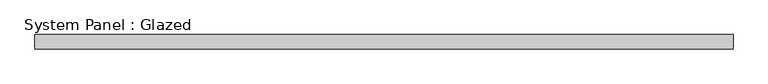
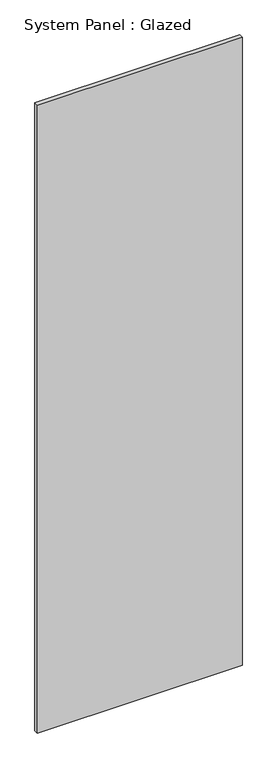
"""IFC4 building model written with IfcOpenShell, lengths in millimetres: plate geometry, System Panel : Glazed."""

from ifc_helpers import new_model, si_unit, origin, origin_with_axes, place, context, project, spatial, polyline, outline, extrude, source, transform, mapped, element, save


def system_panel_glazed_716fcd61(model_context):
    return source(origin(), model_context, "Body", "SweptSolid", [
        extrude(outline(polyline([(622.3, 19.05), (-622.3, 19.05), (-622.3, 44.45), (622.3, 44.45), (622.3, 19.05)])), origin_with_axes(), (0.0, 0.0, 1.0), 4036.0986763),
    ])


if __name__ == "__main__":
    model = new_model("IFC4")
    model_context = context("Model", 3, world=origin())
    ifc_project = project(units=[si_unit("LENGTHUNIT", "METRE", prefix="MILLI")], contexts=[model_context])
    site = spatial("IfcSite", under=ifc_project)
    building = spatial("IfcBuilding", under=site)
    placement = place(None, origin())
    system_panel_glazed_shape = system_panel_glazed_716fcd61(model_context)
    element("IfcPlate", 1, ObjectType="System Panel : Glazed", at=placement, inside=building, context=model_context, shape_type="MappedRepresentation", body=[
        mapped(system_panel_glazed_shape, transform((0.0, 0.0, 0.0), x_axis=(1.0, 0.0, 0.0), y_axis=(0.0, 1.0, 0.0), z_axis=(0.0, 0.0, 1.0))),
    ])
    save(model, "model.ifc")

# Revit data of these elements
# Type "System Panel : Glazed"
#   Construction Type Id = "GSP4R"
#   Analytic Construction = "1/8 in Pilkington single glazing"
#   Visual Light Transmittance = 0.9
#   Solar Heat Gain Coefficient = 0.86
#   Heat Transfer Coefficient (U) = 1.18115 BTU/(h·ft²·°F)
#   Define Thermal Properties by = 1
# Element 1 (IfcPlate, "System Panel : Glazed")
#   Materials on its faces: "Glass"
# Materials
#   "Glass": class "Glass", colour RGB 0 128 192, transparency 0.75, Description = "Soda Lime Glass", Cost = 0
